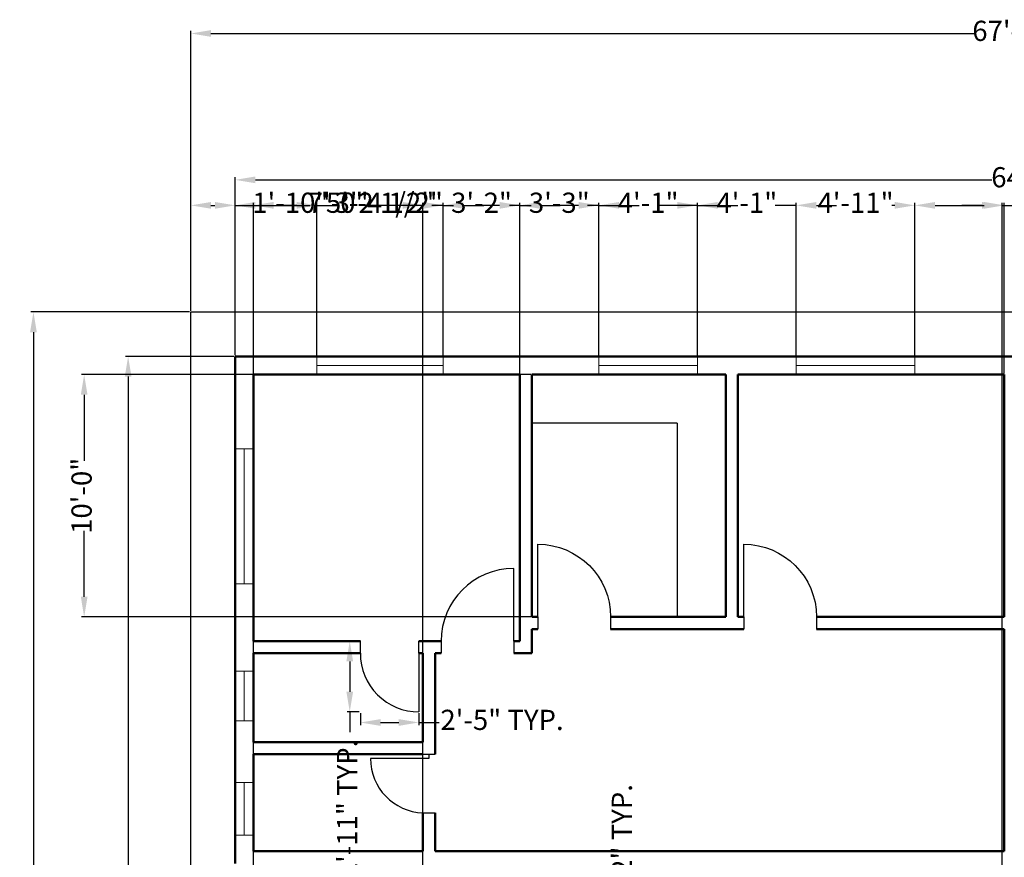
# Model space of a CAD drawing. Units: inches. Extents: x 3237 to 4201, y 2949 to 4053.
# Tile 4 of 5: x 3237 to 3725, y 3638 to 4053. Entities that reach past the tile are written whole.
import ezdxf

# ---------------------------------------------------------------- set-up
doc = ezdxf.new("R2010")
doc.units = ezdxf.units.IN
for name, color, linetype, lineweight in [('A-ANNO-DIMS', 2, 'Continuous', 18), ('A-DOOR', 3, 'Continuous', 25), ('A-FLOR-CASE', 8, 'Continuous', 25), ('A-GLAZ', 4, 'Continuous', 18), ('A-WALL', 7, 'Continuous', 50), ('C-PROP', 6, 'Continuous', 25)]:
    doc.layers.add(name, color=color, linetype=linetype, lineweight=lineweight)
doc.styles.get("Standard").update_dxf_attribs({"font": 'arial.ttf'})
doc.dimstyles.new('ISO-25', dxfattribs={"dimtxt": 10, "dimasz": 10, "dimexe": 1.25, "dimexo": 0.625, "dimtad": 0, "dimdec": 0, "dimlunit": 3, "dimtxsty": 'Standard', "dimcen": 2.5, "dimadec": 0, "dimazin": 0, "dimtfac": 1, "dimtdec": 0, "dimtmove": 0, "dimatfit": 3, "dimfxl": 1, "dimarcsym": 0})

# ---------------------------------------------------------------- blocks, each defined once
blk = doc.blocks.new('*D1')
at = {"layer": 'A-ANNO-DIMS', "color": 0, "lineweight": -2, "transparency": 16777216}
for p, q in [((3321.52, 3908.6), (3321.52, 4047.14)), ((3331.52, 4045.89), (3709.69, 4045.89)), ((4123.52, 4045.89), (3745.35, 4045.89)), ((4133.52, 3908.6), (4133.52, 4047.14))]:
    blk.add_line(p, q, dxfattribs=at)
at = {"layer": 'A-ANNO-DIMS', "color": 0, "transparency": 16777216}
for points in [[(3331.52, 4047.56), (3331.52, 4044.22), (3321.52, 4045.89)], [(4123.52, 4047.56), (4123.52, 4044.22), (4133.52, 4045.89)]]:
    blk.add_solid(points, dxfattribs=at)
at = {"layer": 'Defpoints', "color": 0, "transparency": 16777216}
for p in [(4133.52, 4045.89), (3321.52, 3907.98), (4133.52, 3907.98)]:
    blk.add_point(p, dxfattribs=at)
at = {"layer": 'A-ANNO-DIMS', "color": 0, "transparency": 16777216, "insert": (3727.52, 4045.89), "char_height": 10, "attachment_point": 5}
blk.add_mtext('67\'-8"', dxfattribs=at)
blk = doc.blocks.new('*D2')
at = {"layer": 'A-ANNO-DIMS', "color": 0, "lineweight": -2, "transparency": 16777216}
for p, q in [((3320.9, 3907.98), (3242.34, 3907.98)), ((3243.59, 3897.98), (3243.59, 3467.05)), ((3243.59, 3017.98), (3243.59, 3448.91)), ((3320.9, 3007.98), (3242.34, 3007.98))]:
    blk.add_line(p, q, dxfattribs=at)
at = {"layer": 'A-ANNO-DIMS', "color": 0, "transparency": 16777216}
for points in [[(3241.92, 3897.98), (3245.26, 3897.98), (3243.59, 3907.98)], [(3241.92, 3017.98), (3245.26, 3017.98), (3243.59, 3007.98)]]:
    blk.add_solid(points, dxfattribs=at)
at = {"layer": 'Defpoints', "color": 0, "transparency": 16777216}
for p in [(3321.52, 3907.98), (3243.59, 3007.98), (3321.52, 3007.98)]:
    blk.add_point(p, dxfattribs=at)
at = {"layer": 'A-ANNO-DIMS', "color": 0, "transparency": 16777216, "insert": (3243.59, 3457.98), "char_height": 10, "attachment_point": 5, "rotation": 90}
blk.add_mtext("75'", dxfattribs=at)
blk = doc.blocks.new('*D3')
at = {"layer": 'A-ANNO-DIMS', "color": 0, "lineweight": -2, "transparency": 16777216}
for p, q in [((3343.52, 3886.6), (3343.52, 3974.66)), ((3353.52, 3973.41), (3718.38, 3973.41)), ((4101.52, 3973.41), (3736.66, 3973.41)), ((4111.52, 3886.6), (4111.52, 3974.66))]:
    blk.add_line(p, q, dxfattribs=at)
at = {"layer": 'A-ANNO-DIMS', "color": 0, "transparency": 16777216}
for points in [[(3353.52, 3975.08), (3353.52, 3971.74), (3343.52, 3973.41)], [(4101.52, 3975.08), (4101.52, 3971.74), (4111.52, 3973.41)]]:
    blk.add_solid(points, dxfattribs=at)
at = {"layer": 'Defpoints', "color": 0, "transparency": 16777216}
for p in [(4111.52, 3973.41), (3343.52, 3885.98), (4111.52, 3885.98)]:
    blk.add_point(p, dxfattribs=at)
at = {"layer": 'A-ANNO-DIMS', "color": 0, "transparency": 16777216, "insert": (3727.52, 3973.41), "char_height": 10, "attachment_point": 5}
blk.add_mtext("64'", dxfattribs=at)
blk = doc.blocks.new('*D4')
at = {"layer": 'A-ANNO-DIMS', "color": 0, "lineweight": -2, "transparency": 16777216}
for p, q in [((3342.9, 3885.98), (3289.25, 3885.98)), ((3290.5, 3875.98), (3290.5, 3497.31)), ((3290.5, 3082.98), (3290.5, 3461.65)), ((3342.9, 3072.98), (3289.25, 3072.98))]:
    blk.add_line(p, q, dxfattribs=at)
at = {"layer": 'A-ANNO-DIMS', "color": 0, "transparency": 16777216}
for points in [[(3288.84, 3875.98), (3292.17, 3875.98), (3290.5, 3885.98)], [(3288.84, 3082.98), (3292.17, 3082.98), (3290.5, 3072.98)]]:
    blk.add_solid(points, dxfattribs=at)
at = {"layer": 'Defpoints', "color": 0, "transparency": 16777216}
for p in [(3343.52, 3885.98), (3290.5, 3072.98), (3343.52, 3072.98)]:
    blk.add_point(p, dxfattribs=at)
at = {"layer": 'A-ANNO-DIMS', "color": 0, "transparency": 16777216, "insert": (3290.5, 3479.48), "char_height": 10, "attachment_point": 5, "rotation": 90}
blk.add_mtext('67\'-9"', dxfattribs=at)
blk = doc.blocks.new('DOOR-29-OFFSET-A')
for p, q in [((0, 26), (0, 32)), ((29, 26), (29, 32)), ((0, 29), (2, 29)), ((2, 29), (2, 0))]:
    blk.add_line(p, q)
blk.add_arc((2, 27.02), 27.02, 270, 357.8382)
blk = doc.blocks.new('DOOR-36')
for p, q in [((36, 6), (36, 42)), ((0, 6), (0, 0)), ((36, 6), (36, 0))]:
    blk.add_line(p, q)
blk.add_arc((36, 6), 36, 90, 180)
blk = doc.blocks.new('DOOR-29')
for p, q in [((6, 29), (0, 29)), ((6, 29), (35, 29)), ((6, 0), (0, 0))]:
    blk.add_line(p, q)
blk.add_arc((6, 29), 29, 270, 0)
blk = doc.blocks.new('WIN-66p71IN')
for p, q in [((0, 66.71), (9, 66.71)), ((4.5, 0), (4.5, 66.71)), ((0, 0), (9, 0))]:
    blk.add_line(p, q)
blk = doc.blocks.new('*D17')
at = {"layer": 'A-ANNO-DIMS', "color": 0, "lineweight": -2, "transparency": 16777216}
for p, q in [((3536.36, 3523.25), (3536.36, 3533.25)), ((3532.15, 3523.25), (3537.61, 3523.25)), ((3536.36, 3500.98), (3536.36, 3513.25)), ((3532.15, 3490.98), (3537.61, 3490.98))]:
    blk.add_line(p, q, dxfattribs=at)
at = {"layer": 'A-ANNO-DIMS', "color": 0, "transparency": 16777216}
for points in [[(3534.7, 3513.25), (3538.03, 3513.25), (3536.36, 3523.25)], [(3534.7, 3500.98), (3538.03, 3500.98), (3536.36, 3490.98)]]:
    blk.add_solid(points, dxfattribs=at)
at = {"layer": 'Defpoints', "color": 0, "transparency": 16777216}
for p in [(3531.52, 3523.25), (3536.36, 3523.25), (3531.52, 3490.98)]:
    blk.add_point(p, dxfattribs=at)
at = {"layer": 'A-ANNO-DIMS', "color": 0, "transparency": 16777216, "insert": (3536.36, 3605.25), "char_height": 10, "attachment_point": 5, "rotation": 90}
blk.add_mtext('DOOR B 2\'-8 1/2" TYP.', dxfattribs=at)
blk = doc.blocks.new('*D19')
at = {"layer": 'A-ANNO-DIMS', "color": 0, "lineweight": -2, "transparency": 16777216}
for p, q in [((3404.9, 3744.98), (3399.02, 3744.98)), ((3400.27, 3734.98), (3400.27, 3719.98)), ((3404.9, 3709.98), (3399.02, 3709.98)), ((3400.27, 3709.98), (3400.27, 3699.98))]:
    blk.add_line(p, q, dxfattribs=at)
at = {"layer": 'A-ANNO-DIMS', "color": 0, "transparency": 16777216}
for points in [[(3398.61, 3734.98), (3401.94, 3734.98), (3400.27, 3744.98)], [(3398.61, 3719.98), (3401.94, 3719.98), (3400.27, 3709.98)]]:
    blk.add_solid(points, dxfattribs=at)
at = {"layer": 'Defpoints', "color": 0, "transparency": 16777216}
for p in [(3405.52, 3744.98), (3400.27, 3709.98), (3405.52, 3709.98)]:
    blk.add_point(p, dxfattribs=at)
at = {"layer": 'A-ANNO-DIMS', "color": 0, "transparency": 16777216, "insert": (3400.27, 3635.36), "char_height": 10, "attachment_point": 5, "rotation": 90}
blk.add_mtext('DOOR C 2\'-11" TYP.', dxfattribs=at)
blk = doc.blocks.new('*D20')
at = {"layer": 'A-ANNO-DIMS', "color": 0, "lineweight": -2, "transparency": 16777216}
for p, q in [((3405.52, 3709.35), (3405.52, 3703.48)), ((3434.52, 3709.35), (3434.52, 3703.48)), ((3415.52, 3704.73), (3424.52, 3704.73)), ((3434.52, 3704.73), (3444.52, 3704.73))]:
    blk.add_line(p, q, dxfattribs=at)
at = {"layer": 'A-ANNO-DIMS', "color": 0, "transparency": 16777216}
for points in [[(3415.52, 3706.4), (3415.52, 3703.06), (3405.52, 3704.73)], [(3424.52, 3706.4), (3424.52, 3703.06), (3434.52, 3704.73)]]:
    blk.add_solid(points, dxfattribs=at)
at = {"layer": 'Defpoints', "color": 0, "transparency": 16777216}
for p in [(3405.52, 3709.98), (3434.52, 3709.98), (3434.52, 3704.73)]:
    blk.add_point(p, dxfattribs=at)
at = {"layer": 'A-ANNO-DIMS', "color": 0, "transparency": 16777216, "insert": (3475.71, 3704.73), "char_height": 10, "attachment_point": 5}
blk.add_mtext('2\'-5" TYP.', dxfattribs=at)
blk = doc.blocks.new('*D35')
at = {"layer": 'A-ANNO-DIMS', "color": 0, "lineweight": -2, "transparency": 16777216}
for p, q in [((3343.52, 3886.6), (3343.52, 3962.03)), ((3353.52, 3960.78), (3374.01, 3960.78)), ((3384.01, 3886.6), (3384.01, 3962.03)), ((3384.01, 3960.78), (3394.01, 3960.78))]:
    blk.add_line(p, q, dxfattribs=at)
at = {"layer": 'A-ANNO-DIMS', "color": 0, "transparency": 16777216}
for points in [[(3353.52, 3962.45), (3353.52, 3959.11), (3343.52, 3960.78)], [(3374.01, 3962.45), (3374.01, 3959.11), (3384.01, 3960.78)]]:
    blk.add_solid(points, dxfattribs=at)
at = {"layer": 'Defpoints', "color": 0, "transparency": 16777216}
for p in [(3384.01, 3960.78), (3343.52, 3885.98), (3384.01, 3885.98)]:
    blk.add_point(p, dxfattribs=at)
at = {"layer": 'A-ANNO-DIMS', "color": 0, "transparency": 16777216, "insert": (3419.58, 3960.78), "char_height": 10, "attachment_point": 5}
blk.add_mtext('3\'-4 1/2"', dxfattribs=at)
blk = doc.blocks.new('*D36')
at = {"layer": 'A-ANNO-DIMS', "color": 0, "lineweight": -2, "transparency": 16777216}
for p, q in [((3374.01, 3960.78), (3364.01, 3960.78)), ((3384.01, 3886.6), (3384.01, 3962.03)), ((3384.01, 3960.78), (3389.75, 3960.78)), ((3446.62, 3960.78), (3440.88, 3960.78)), ((3446.62, 3886.6), (3446.62, 3962.03)), ((3456.62, 3960.78), (3466.62, 3960.78))]:
    blk.add_line(p, q, dxfattribs=at)
at = {"layer": 'A-ANNO-DIMS', "color": 0, "transparency": 16777216}
for points in [[(3374.01, 3962.45), (3374.01, 3959.11), (3384.01, 3960.78)], [(3456.62, 3962.45), (3456.62, 3959.11), (3446.62, 3960.78)]]:
    blk.add_solid(points, dxfattribs=at)
at = {"layer": 'Defpoints', "color": 0, "transparency": 16777216}
for p in [(3446.62, 3960.78), (3384.01, 3885.98), (3446.62, 3885.98)]:
    blk.add_point(p, dxfattribs=at)
at = {"layer": 'A-ANNO-DIMS', "color": 0, "transparency": 16777216, "insert": (3415.32, 3960.78), "char_height": 10, "attachment_point": 5}
blk.add_mtext('5\'-2 1/2"', dxfattribs=at)
blk = doc.blocks.new('*D37')
at = {"layer": 'A-ANNO-DIMS', "color": 0, "lineweight": -2, "transparency": 16777216}
for p, q in [((3436.62, 3960.78), (3426.62, 3960.78)), ((3446.62, 3886.6), (3446.62, 3962.03)), ((3446.62, 3960.78), (3451.66, 3960.78)), ((3484.52, 3960.78), (3479.48, 3960.78)), ((3484.52, 3877.6), (3484.52, 3962.03)), ((3494.52, 3960.78), (3504.52, 3960.78))]:
    blk.add_line(p, q, dxfattribs=at)
at = {"layer": 'A-ANNO-DIMS', "color": 0, "transparency": 16777216}
for points in [[(3436.62, 3962.45), (3436.62, 3959.11), (3446.62, 3960.78)], [(3494.52, 3962.45), (3494.52, 3959.11), (3484.52, 3960.78)]]:
    blk.add_solid(points, dxfattribs=at)
at = {"layer": 'Defpoints', "color": 0, "transparency": 16777216}
for p in [(3484.52, 3960.78), (3446.62, 3885.98), (3484.52, 3876.98)]:
    blk.add_point(p, dxfattribs=at)
at = {"layer": 'A-ANNO-DIMS', "color": 0, "transparency": 16777216, "insert": (3465.57, 3960.78), "char_height": 10, "attachment_point": 5}
blk.add_mtext('3\'-2"', dxfattribs=at)
blk = doc.blocks.new('*D38')
at = {"layer": 'A-ANNO-DIMS', "color": 0, "lineweight": -2, "transparency": 16777216}
for p, q in [((3474.52, 3960.78), (3464.52, 3960.78)), ((3484.52, 3877.6), (3484.52, 3962.03)), ((3484.52, 3960.78), (3490.16, 3960.78)), ((3523.63, 3960.78), (3517.99, 3960.78)), ((3523.63, 3886.6), (3523.63, 3962.03)), ((3533.63, 3960.78), (3543.63, 3960.78))]:
    blk.add_line(p, q, dxfattribs=at)
at = {"layer": 'A-ANNO-DIMS', "color": 0, "transparency": 16777216}
for points in [[(3474.52, 3962.45), (3474.52, 3959.11), (3484.52, 3960.78)], [(3533.63, 3962.45), (3533.63, 3959.11), (3523.63, 3960.78)]]:
    blk.add_solid(points, dxfattribs=at)
at = {"layer": 'Defpoints', "color": 0, "transparency": 16777216}
for p in [(3523.63, 3960.78), (3523.63, 3885.98), (3484.52, 3876.98)]:
    blk.add_point(p, dxfattribs=at)
at = {"layer": 'A-ANNO-DIMS', "color": 0, "transparency": 16777216, "insert": (3504.08, 3960.78), "char_height": 10, "attachment_point": 5}
blk.add_mtext('3\'-3"', dxfattribs=at)
blk = doc.blocks.new('*D39')
at = {"layer": 'A-ANNO-DIMS', "color": 0, "lineweight": -2, "transparency": 16777216}
for p, q in [((3513.63, 3960.78), (3503.63, 3960.78)), ((3523.63, 3886.6), (3523.63, 3962.03)), ((3523.63, 3960.78), (3533.96, 3960.78)), ((3572.52, 3960.78), (3562.19, 3960.78)), ((3572.52, 3886.6), (3572.52, 3962.03)), ((3582.52, 3960.78), (3592.52, 3960.78))]:
    blk.add_line(p, q, dxfattribs=at)
at = {"layer": 'A-ANNO-DIMS', "color": 0, "transparency": 16777216}
for points in [[(3513.63, 3962.45), (3513.63, 3959.11), (3523.63, 3960.78)], [(3582.52, 3962.45), (3582.52, 3959.11), (3572.52, 3960.78)]]:
    blk.add_solid(points, dxfattribs=at)
at = {"layer": 'Defpoints', "color": 0, "transparency": 16777216}
for p in [(3572.52, 3960.78), (3523.63, 3885.98), (3572.52, 3885.98)]:
    blk.add_point(p, dxfattribs=at)
at = {"layer": 'A-ANNO-DIMS', "color": 0, "transparency": 16777216, "insert": (3548.08, 3960.78), "char_height": 10, "attachment_point": 5}
blk.add_mtext('4\'-1"', dxfattribs=at)
blk = doc.blocks.new('*D40')
at = {"layer": 'A-ANNO-DIMS', "color": 0, "lineweight": -2, "transparency": 16777216}
for p, q in [((3562.52, 3960.78), (3552.52, 3960.78)), ((3572.52, 3886.6), (3572.52, 3962.03)), ((3572.52, 3960.78), (3582.86, 3960.78)), ((3621.43, 3960.78), (3611.09, 3960.78)), ((3621.43, 3886.6), (3621.43, 3962.03)), ((3631.43, 3960.78), (3641.43, 3960.78))]:
    blk.add_line(p, q, dxfattribs=at)
at = {"layer": 'A-ANNO-DIMS', "color": 0, "transparency": 16777216}
for points in [[(3562.52, 3962.45), (3562.52, 3959.11), (3572.52, 3960.78)], [(3631.43, 3962.45), (3631.43, 3959.11), (3621.43, 3960.78)]]:
    blk.add_solid(points, dxfattribs=at)
at = {"layer": 'Defpoints', "color": 0, "transparency": 16777216}
for p in [(3621.43, 3960.78), (3572.52, 3885.98), (3621.43, 3885.98)]:
    blk.add_point(p, dxfattribs=at)
at = {"layer": 'A-ANNO-DIMS', "color": 0, "transparency": 16777216, "insert": (3596.98, 3960.78), "char_height": 10, "attachment_point": 5}
blk.add_mtext('4\'-1"', dxfattribs=at)
blk = doc.blocks.new('*D41')
at = {"layer": 'A-ANNO-DIMS', "color": 0, "lineweight": -2, "transparency": 16777216}
for p, q in [((3621.43, 3886.6), (3621.43, 3962.03)), ((3631.43, 3960.78), (3632.84, 3960.78)), ((3670.25, 3960.78), (3668.84, 3960.78)), ((3680.25, 3886.6), (3680.25, 3962.03))]:
    blk.add_line(p, q, dxfattribs=at)
at = {"layer": 'A-ANNO-DIMS', "color": 0, "transparency": 16777216}
for points in [[(3631.43, 3962.45), (3631.43, 3959.11), (3621.43, 3960.78)], [(3670.25, 3962.45), (3670.25, 3959.11), (3680.25, 3960.78)]]:
    blk.add_solid(points, dxfattribs=at)
at = {"layer": 'Defpoints', "color": 0, "transparency": 16777216}
for p in [(3680.25, 3960.78), (3621.43, 3885.98), (3680.25, 3885.98)]:
    blk.add_point(p, dxfattribs=at)
at = {"layer": 'A-ANNO-DIMS', "color": 0, "transparency": 16777216, "insert": (3650.84, 3960.78), "char_height": 10, "attachment_point": 5}
blk.add_mtext('4\'-11"', dxfattribs=at)
blk = doc.blocks.new('*D42')
at = {"layer": 'A-ANNO-DIMS', "color": 0, "lineweight": -2, "transparency": 16777216}
for p, q in [((3680.25, 3886.6), (3680.25, 3962.03)), ((3690.25, 3960.78), (3714.52, 3960.78)), ((3724.52, 3877.6), (3724.52, 3962.03)), ((3724.52, 3960.78), (3734.52, 3960.78))]:
    blk.add_line(p, q, dxfattribs=at)
at = {"layer": 'A-ANNO-DIMS', "color": 0, "transparency": 16777216}
for points in [[(3690.25, 3962.45), (3690.25, 3959.11), (3680.25, 3960.78)], [(3714.52, 3962.45), (3714.52, 3959.11), (3724.52, 3960.78)]]:
    blk.add_solid(points, dxfattribs=at)
at = {"layer": 'Defpoints', "color": 0, "transparency": 16777216}
for p in [(3724.52, 3960.78), (3680.25, 3885.98), (3724.52, 3876.98)]:
    blk.add_point(p, dxfattribs=at)
at = {"layer": 'A-ANNO-DIMS', "color": 0, "transparency": 16777216, "insert": (3760.09, 3960.78), "char_height": 10, "attachment_point": 5}
blk.add_mtext('3\'-8 1/2"', dxfattribs=at)
blk = doc.blocks.new('*D51')
at = {"layer": 'A-ANNO-DIMS', "color": 0, "lineweight": -2, "transparency": 16777216}
for p, q in [((3321.52, 3908.6), (3321.52, 3962.03)), ((3331.52, 3960.78), (3333.52, 3960.78)), ((3343.52, 3886.6), (3343.52, 3962.03)), ((3343.52, 3960.78), (3353.52, 3960.78))]:
    blk.add_line(p, q, dxfattribs=at)
at = {"layer": 'A-ANNO-DIMS', "color": 0, "transparency": 16777216}
for points in [[(3331.52, 3962.45), (3331.52, 3959.11), (3321.52, 3960.78)], [(3333.52, 3962.45), (3333.52, 3959.11), (3343.52, 3960.78)]]:
    blk.add_solid(points, dxfattribs=at)
at = {"layer": 'Defpoints', "color": 0, "transparency": 16777216}
for p in [(3343.52, 3960.78), (3321.52, 3907.98), (3343.52, 3885.98)]:
    blk.add_point(p, dxfattribs=at)
at = {"layer": 'A-ANNO-DIMS', "color": 0, "transparency": 16777216, "insert": (3370.85, 3960.78), "char_height": 10, "attachment_point": 5}
blk.add_mtext('1\'-10"', dxfattribs=at)
blk = doc.blocks.new('*D69')
at = {"layer": 'A-ANNO-DIMS', "color": 0, "lineweight": -2, "transparency": 16777216}
for p, q in [((3489.9, 3876.98), (3267.47, 3876.98)), ((3268.72, 3866.98), (3268.72, 3834.31)), ((3268.72, 3766.98), (3268.72, 3799.65)), ((3489.9, 3756.98), (3267.47, 3756.98))]:
    blk.add_line(p, q, dxfattribs=at)
at = {"layer": 'A-ANNO-DIMS', "color": 0, "transparency": 16777216}
for points in [[(3267.06, 3866.98), (3270.39, 3866.98), (3268.72, 3876.98)], [(3267.06, 3766.98), (3270.39, 3766.98), (3268.72, 3756.98)]]:
    blk.add_solid(points, dxfattribs=at)
at = {"layer": 'Defpoints', "color": 0, "transparency": 16777216}
for p in [(3268.72, 3876.98), (3490.52, 3876.98), (3490.52, 3756.98)]:
    blk.add_point(p, dxfattribs=at)
at = {"layer": 'A-ANNO-DIMS', "color": 0, "transparency": 16777216, "insert": (3268.72, 3816.98), "char_height": 10, "attachment_point": 5, "rotation": 90}
blk.add_mtext('10\'-0"', dxfattribs=at)
blk = doc.blocks.new('*D73')
at = {"layer": 'A-ANNO-DIMS', "color": 0, "lineweight": -2, "transparency": 16777216}
for p, q in [((3352.52, 3329.6), (3352.52, 3962.03)), ((3362.52, 3960.78), (3380.65, 3960.78)), ((3426.52, 3960.78), (3408.4, 3960.78)), ((3436.52, 3329.6), (3436.52, 3962.03))]:
    blk.add_line(p, q, dxfattribs=at)
at = {"layer": 'A-ANNO-DIMS', "color": 0, "transparency": 16777216}
for points in [[(3362.52, 3962.45), (3362.52, 3959.11), (3352.52, 3960.78)], [(3426.52, 3962.45), (3426.52, 3959.11), (3436.52, 3960.78)]]:
    blk.add_solid(points, dxfattribs=at)
at = {"layer": 'Defpoints', "color": 0, "transparency": 16777216}
for p in [(3436.52, 3960.78), (3352.52, 3328.98), (3436.52, 3328.98)]:
    blk.add_point(p, dxfattribs=at)
at = {"layer": 'A-ANNO-DIMS', "color": 0, "transparency": 16777216, "insert": (3394.52, 3960.78), "char_height": 10, "attachment_point": 5}
blk.add_mtext('7\'-0"', dxfattribs=at)
blk = doc.blocks.new('*D83')
at = {"layer": 'A-ANNO-DIMS', "color": 0, "lineweight": -2, "transparency": 16777216}
for p, q in [((3713.52, 3960.78), (3703.52, 3960.78)), ((3723.52, 3193.4), (3723.52, 3962.03)), ((3723.52, 3960.78), (3733.4, 3960.78)), ((3771.52, 3960.78), (3761.64, 3960.78)), ((3771.52, 3193.4), (3771.52, 3962.03)), ((3781.52, 3960.78), (3791.52, 3960.78))]:
    blk.add_line(p, q, dxfattribs=at)
at = {"layer": 'A-ANNO-DIMS', "color": 0, "transparency": 16777216}
for points in [[(3713.52, 3962.45), (3713.52, 3959.11), (3723.52, 3960.78)], [(3781.52, 3962.45), (3781.52, 3959.11), (3771.52, 3960.78)]]:
    blk.add_solid(points, dxfattribs=at)
at = {"layer": 'Defpoints', "color": 0, "transparency": 16777216}
for p in [(3771.52, 3960.78), (3723.52, 3192.78), (3771.52, 3192.78)]:
    blk.add_point(p, dxfattribs=at)
at = {"layer": 'A-ANNO-DIMS', "color": 0, "transparency": 16777216, "insert": (3747.52, 3960.78), "char_height": 10, "attachment_point": 5}
blk.add_mtext('4\'-0"', dxfattribs=at)

msp = doc.modelspace()

# ---------------------------------------------------------------- linework, layer by layer
at = {"layer": 'A-FLOR-CASE'}
for q in [(3490.52, 3852.98), (3562.52, 3756.98)]:
    msp.add_line((3562.52, 3852.98), q, dxfattribs=at)
at = {"layer": 'A-GLAZ'}
for p, q in [((3384.01, 3876.98), (3384.01, 3885.98)), ((3446.62, 3876.98), (3446.62, 3885.98)), ((3523.63, 3876.98), (3523.63, 3885.98)), ((3572.52, 3876.98), (3572.52, 3885.98)), ((3621.43, 3876.98), (3621.43, 3885.98)), ((3680.25, 3876.98), (3680.25, 3885.98)), ((3384.01, 3881.48), (3446.62, 3881.48)), ((3523.63, 3881.48), (3572.52, 3881.48)), ((3680.25, 3881.48), (3621.43, 3881.48)), ((3343.52, 3773.45), (3343.52, 3840.16)), ((3352.52, 3730.16), (3343.52, 3730.16)), ((3348.02, 3730.16), (3348.02, 3705.54)), ((3352.52, 3705.54), (3343.52, 3705.54)), ((3352.52, 3674.94), (3343.52, 3674.94)), ((3348.02, 3674.94), (3348.02, 3648.9)), ((3352.52, 3648.9), (3343.52, 3648.9))]:
    msp.add_line(p, q, dxfattribs=at)
at = {"layer": 'A-WALL'}
for p, q in [((4111.52, 3885.98), (3343.52, 3885.98)), ((3343.52, 3885.98), (3343.52, 3634.98)), ((3352.52, 3876.98), (3352.52, 3744.98)), ((3484.52, 3876.98), (3352.52, 3876.98)), ((3484.52, 3876.98), (3484.52, 3744.98)), ((3490.52, 3876.98), (3490.52, 3756.98)), ((3586.52, 3876.98), (3490.52, 3876.98)), ((3586.52, 3876.98), (3586.52, 3756.98)), ((3592.52, 3876.98), (3592.52, 3756.98)), ((3724.52, 3876.98), (3592.52, 3876.98)), ((3724.52, 3876.98), (3724.52, 3756.98)), ((3493.52, 3756.98), (3490.52, 3756.98)), ((3586.52, 3756.98), (3529.52, 3756.98)), ((3595.52, 3756.98), (3592.52, 3756.98)), ((3724.52, 3756.98), (3631.52, 3756.98)), ((3490.52, 3750.98), (3490.52, 3738.98)), ((3493.52, 3750.98), (3490.52, 3750.98)), ((3595.52, 3750.98), (3529.52, 3750.98)), ((3724.52, 3750.98), (3631.52, 3750.98)), ((3724.52, 3750.98), (3724.52, 3640.98)), ((3405.52, 3744.98), (3352.52, 3744.98)), ((3445.52, 3744.98), (3434.52, 3744.98)), ((3484.52, 3744.98), (3481.52, 3744.98)), ((3352.52, 3738.98), (3352.52, 3694.98)), ((3405.52, 3738.98), (3352.52, 3738.98)), ((3436.52, 3738.98), (3434.52, 3738.98)), ((3436.52, 3738.98), (3436.52, 3694.98)), ((3442.52, 3738.98), (3442.52, 3688.98)), ((3445.52, 3738.98), (3442.52, 3738.98)), ((3490.52, 3738.98), (3481.52, 3738.98)), ((3436.52, 3694.98), (3352.52, 3694.98)), ((3436.52, 3688.98), (3352.52, 3688.98)), ((3352.52, 3688.98), (3352.52, 3640.98)), ((3436.52, 3659.98), (3436.52, 3640.98)), ((3442.52, 3659.98), (3442.52, 3640.98)), ((3436.52, 3640.98), (3352.52, 3640.98)), ((3490.52, 3640.98), (3442.52, 3640.98)), ((3724.52, 3640.98), (3484.52, 3640.98))]:
    msp.add_line(p, q, dxfattribs=at)
at = {"layer": 'C-PROP'}
for p, q in [((3321.52, 3007.98), (3321.52, 3907.98)), ((3321.52, 3907.98), (4133.52, 3907.98))]:
    msp.add_line(p, q, dxfattribs=at)

# ---------------------------------------------------------------- block references
at = {"layer": 'A-DOOR', "extrusion": (0, 0, -1), "zscale": -1}
for p in [(-3529.52, 3750.98), (-3631.52, 3750.98)]:
    msp.add_blockref('DOOR-36', p, dxfattribs=at)
at = {"layer": 'A-DOOR'}
msp.add_blockref('DOOR-36', (3445.52, 3738.98), dxfattribs=at)
for name, p, rotation in [('DOOR-29', (3405.52, 3744.98), 269.9999999999989), ('DOOR-29-OFFSET-A', (3410.52, 3688.98), 270.0000000000055)]:
    msp.add_blockref(name, p, dxfattribs=dict(at, rotation=rotation))
at = {"layer": 'A-GLAZ'}
msp.add_blockref('WIN-66p71IN', (3343.52, 3773.45), dxfattribs=at)

# ---------------------------------------------------------------- dimensions: what is measured, and where the dimension line sits
at = {"layer": 'A-ANNO-DIMS'}
for base, p1, p2, override, picture, middle in [((4133.52, 4045.89), (3321.52, 3907.98), (4133.52, 3907.98), {"dimclrd": 0, "dimclre": 0, "dimclrt": 0}, '*D1', (3727.52, 4045.89)), ((4111.52, 3973.41), (3343.52, 3885.98), (4111.52, 3885.98), {"dimclrd": 0, "dimclre": 0, "dimclrt": 0}, '*D3', (3727.52, 3973.41)), ((3384.01, 3960.78), (3343.52, 3885.98), (3384.01, 3885.98), {"dimdec": 1, "dimlfac": 1, "dimrnd": 0, "dimzin": 1, "dimdsep": 46, "dimlunit": 4, "dimfrac": 2}, '*D35', (3419.58, 3960.78)), ((3446.62, 3960.78), (3384.01, 3885.98), (3446.62, 3885.98), {"dimdec": 1, "dimlfac": 1, "dimrnd": 0, "dimzin": 1, "dimdsep": 46, "dimlunit": 4, "dimfrac": 2}, '*D36', (3415.32, 3960.78)), ((3724.52, 3960.78), (3680.25, 3885.98), (3724.52, 3876.98), {"dimdec": 1, "dimlfac": 1, "dimrnd": 0, "dimzin": 1, "dimdsep": 46, "dimlunit": 4, "dimfrac": 2}, '*D42', (3760.09, 3960.78)), ((3343.52, 3960.78), (3321.52, 3907.98), (3343.52, 3885.98), {"dimdec": 1, "dimlfac": 1, "dimrnd": 0, "dimzin": 1, "dimdsep": 46, "dimlunit": 4, "dimfrac": 2}, '*D51', (3370.85, 3960.78)), ((3436.52, 3960.78), (3352.52, 3328.98), (3436.52, 3328.98), {"dimdec": 1, "dimlfac": 1, "dimrnd": 0, "dimzin": 1, "dimdsep": 46, "dimlunit": 4, "dimfrac": 2}, '*D73', (3394.52, 3960.78)), ((3484.52, 3960.78), (3446.62, 3885.98), (3484.52, 3876.98), {"dimdec": 1, "dimlfac": 1, "dimrnd": 0, "dimzin": 1, "dimdsep": 46, "dimlunit": 4, "dimfrac": 2}, '*D37', (3465.57, 3960.78)), ((3523.63, 3960.78), (3484.52, 3876.98), (3523.63, 3885.98), {"dimdec": 1, "dimlfac": 1, "dimrnd": 0, "dimzin": 1, "dimdsep": 46, "dimlunit": 4, "dimfrac": 2}, '*D38', (3504.08, 3960.78)), ((3572.52, 3960.78), (3523.63, 3885.98), (3572.52, 3885.98), {"dimdec": 1, "dimlfac": 1, "dimrnd": 0, "dimzin": 1, "dimdsep": 46, "dimlunit": 4, "dimfrac": 2}, '*D39', (3548.08, 3960.78)), ((3621.43, 3960.78), (3572.52, 3885.98), (3621.43, 3885.98), {"dimdec": 1, "dimlfac": 1, "dimrnd": 0, "dimzin": 1, "dimdsep": 46, "dimlunit": 4, "dimfrac": 2}, '*D40', (3596.98, 3960.78)), ((3680.25, 3960.78), (3621.43, 3885.98), (3680.25, 3885.98), {"dimdec": 1, "dimlfac": 1, "dimrnd": 0, "dimzin": 1, "dimdsep": 46, "dimlunit": 4, "dimfrac": 2}, '*D41', (3650.84, 3960.78)), ((3771.52, 3960.78), (3723.52, 3192.78), (3771.52, 3192.78), {"dimdec": 1, "dimlfac": 1, "dimrnd": 0, "dimzin": 1, "dimdsep": 46, "dimlunit": 4, "dimfrac": 2}, '*D83', (3747.52, 3960.78))]:
    dim = msp.add_linear_dim(base=base, p1=p1, p2=p2, dimstyle='ISO-25', override=override, dxfattribs=at)
    dim.commit()
    dim.dimension.update_dxf_attribs({"geometry": picture, "text_midpoint": middle})
for base, p1, p2, override, picture, middle in [((3243.59, 3007.98), (3321.52, 3907.98), (3321.52, 3007.98), {"dimclrd": 0, "dimclre": 0, "dimclrt": 0}, '*D2', (3243.59, 3457.98)), ((3290.5, 3072.98), (3343.52, 3885.98), (3343.52, 3072.98), {"dimclrd": 0, "dimclre": 0, "dimclrt": 0}, '*D4', (3290.5, 3479.48)), ((3268.72, 3876.98), (3490.52, 3756.98), (3490.52, 3876.98), {"dimdec": 1, "dimlfac": 1, "dimrnd": 0, "dimzin": 1, "dimdsep": 46, "dimlunit": 4, "dimfrac": 2}, '*D69', (3268.72, 3816.98))]:
    dim = msp.add_linear_dim(base=base, p1=p1, p2=p2, angle=90, dimstyle='ISO-25', override=override, dxfattribs=at)
    dim.commit()
    dim.dimension.update_dxf_attribs({"geometry": picture, "text_midpoint": middle})
for base, p1, p2, angle, text, picture, middle in [((3400.27, 3709.98), (3405.52, 3744.98), (3405.52, 3709.98), 270, 'DOOR C <> TYP.', '*D19', (3400.27, 3635.36)), ((3536.36, 3523.25), (3531.52, 3490.98), (3531.52, 3523.25), 90, 'DOOR B <> TYP.', '*D17', (3536.36, 3605.25))]:
    dim = msp.add_linear_dim(base=base, p1=p1, p2=p2, angle=angle, text=text, dimstyle='ISO-25', override={"dimdec": 1, "dimlfac": 1, "dimrnd": 0, "dimzin": 1, "dimdsep": 46, "dimlunit": 4, "dimfrac": 2}, dxfattribs=at)
    dim.commit()
    dim.dimension.update_dxf_attribs({"geometry": picture, "text_midpoint": middle})
dim = msp.add_linear_dim(base=(3434.52, 3704.73), p1=(3405.52, 3709.98), p2=(3434.52, 3709.98), text='<> TYP.', dimstyle='ISO-25', override={"dimdec": 1, "dimlfac": 1, "dimrnd": 0, "dimzin": 1, "dimdsep": 46, "dimlunit": 4, "dimfrac": 2}, dxfattribs=at)
dim.commit()
dim.dimension.update_dxf_attribs({"geometry": '*D20', "text_midpoint": (3475.71, 3704.73)})

doc.saveas('drawing.dxf')
